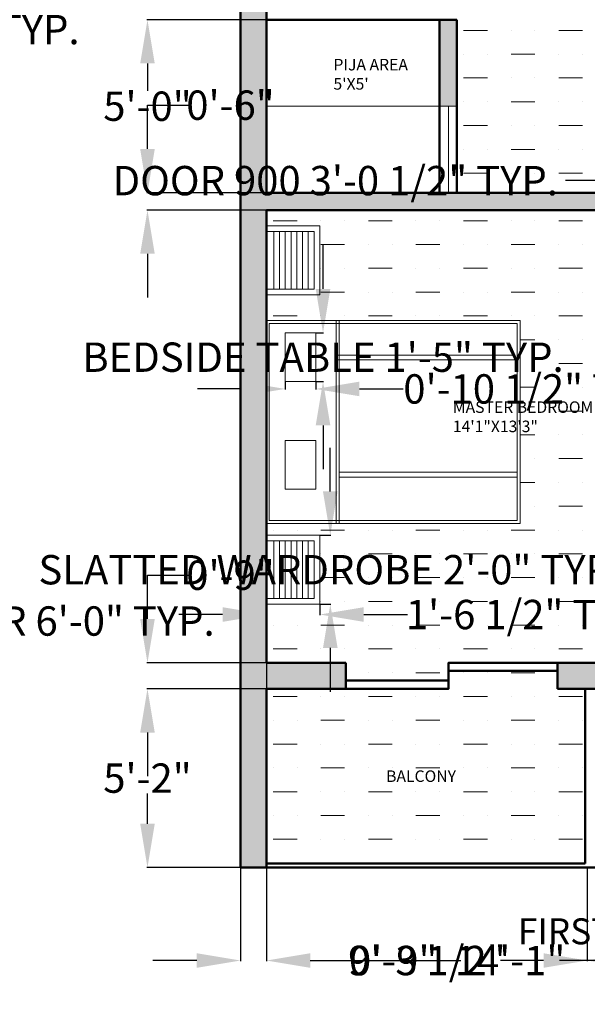
# Model space of a CAD drawing. Units: inches. Extents: x 26 to 14419, y 2 to 3479.
# Tile 6 of 9: x 14003 to 14200, y 2764 to 3106. Entities that reach past the tile are written whole.
import ezdxf

# ---------------------------------------------------------------- set-up
doc = ezdxf.new("R2010")
doc.units = ezdxf.units.IN
doc.header["$MEASUREMENT"] = 0
for name, color, linetype, lineweight in [('A-ANNO-DIMS', 2, 'Continuous', 18), ('A-ANNO-TEXT', 7, 'Continuous', 25), ('A-AREA-IDEN', 7, 'Continuous', 18), ('A-FLOR-PATT', 252, 'Continuous', 13), ('A-FURN', 8, 'Continuous', 18), ('A-WALL', 7, 'Continuous', 50)]:
    doc.layers.add(name, color=color, linetype=linetype, lineweight=lineweight)
doc.styles.get("Standard").update_dxf_attribs({"font": 'arial.ttf'})
doc.dimstyles.get("Standard").update_dxf_attribs({"dimtxt": 10.18, "dimasz": 15.18, "dimexe": 0.18, "dimexo": 0.0625, "dimgap": 0.09, "dimtad": 0, "dimtih": 1, "dimtoh": 1, "dimdec": 0, "dimzin": 0, "dimdsep": 46, "dimlunit": 3, "dimtxsty": 'Standard', "dimcen": 0.09, "dimadec": 0, "dimazin": 0, "dimtfac": 1, "dimtdec": 0, "dimtofl": 0, "dimtmove": 0, "dimatfit": 3, "dimfxl": 1, "dimtolj": 1, "dimtzin": 0, "dimarcsym": 0})

# ---------------------------------------------------------------- blocks, each defined once
blk = doc.blocks.new('WARDROBE-SLAT')
for p, q in [((2.53, 21.91), (2.53, 2)), ((4.53, 21.91), (4.53, 2)), ((6.53, 21.91), (6.53, 2)), ((8.53, 21.91), (8.53, 2)), ((10.53, 21.91), (10.53, 2)), ((12.53, 21.91), (12.53, 2)), ((14.53, 21.91), (14.53, 2))]:
    blk.add_line(p, q)
blk.add_lwpolyline([(0, 23.91), (18.56, 23.91), (18.56, 0), (0, 0)])
blk.add_lwpolyline([(0, 21.91), (16.56, 21.91), (16.56, 2), (0, 2)], close=True)
blk = doc.blocks.new('BEDSIDE-TABLE')
blk.add_lwpolyline([(0, 16.94), (10.58, 16.94), (10.58, 0), (0, 0)], close=True)
blk = doc.blocks.new('*D25')
at = {"layer": 'A-ANNO-DIMS', "color": 0, "lineweight": -2, "transparency": 16777216}
for p, q in [((14212.95, 3101.37), (14207.39, 3101.37)), ((14207.57, 3086.19), (14207.57, 3080.27)), ((14212.95, 3065.09), (14207.39, 3065.09)), ((14207.57, 3065.09), (14207.57, 3049.91)), ((14207.57, 3049.91), (14192.39, 3049.91))]:
    blk.add_line(p, q, dxfattribs=at)
at = {"layer": 'A-ANNO-DIMS', "color": 0, "transparency": 16777216}
for points in [[(14205.04, 3086.19), (14210.1, 3086.19), (14207.57, 3101.37)], [(14205.04, 3080.27), (14210.1, 3080.27), (14207.57, 3065.09)]]:
    blk.add_solid(points, dxfattribs=at)
at = {"layer": 'Defpoints', "color": 0, "transparency": 16777216}
for p in [(14213.01, 3101.37), (14207.57, 3065.09), (14213.01, 3065.09)]:
    blk.add_point(p, dxfattribs=at)
at = {"layer": 'A-ANNO-DIMS', "color": 0, "transparency": 16777216, "insert": (14112.52, 3049.91), "char_height": 10.18, "attachment_point": 5}
blk.add_mtext('\\A1;DOOR 900 3\'-0 1/2" TYP.', dxfattribs=at)
blk = doc.blocks.new('*D29')
at = {"layer": 'A-ANNO-DIMS', "color": 0, "lineweight": -2, "transparency": 16777216}
for p, q in [((13817.09, 2907.93), (13817.09, 2897.02)), ((13889.09, 2907.93), (13889.09, 2897.02)), ((13832.27, 2897.2), (13873.91, 2897.2)), ((13889.09, 2897.2), (13904.27, 2897.2))]:
    blk.add_line(p, q, dxfattribs=at)
at = {"layer": 'A-ANNO-DIMS', "color": 0, "transparency": 16777216}
for points in [[(13832.27, 2899.73), (13832.27, 2894.67), (13817.09, 2897.2)], [(13873.91, 2899.73), (13873.91, 2894.67), (13889.09, 2897.2)]]:
    blk.add_solid(points, dxfattribs=at)
at = {"layer": 'Defpoints', "color": 0, "transparency": 16777216}
for p in [(13817.09, 2908), (13889.09, 2908), (13889.09, 2897.2)]:
    blk.add_point(p, dxfattribs=at)
at = {"layer": 'A-ANNO-DIMS', "color": 0, "transparency": 16777216, "insert": (13989.66, 2897.2), "char_height": 10.18, "attachment_point": 5}
blk.add_mtext('\\A1;DOUBLE DOOR 6\'-0" TYP.', dxfattribs=at)
blk = doc.blocks.new('*D39')
at = {"layer": 'A-ANNO-DIMS', "color": 0, "lineweight": -2, "transparency": 16777216}
for p, q in [((14110.79, 2942.13), (14110.79, 2957.31)), ((14107.27, 2926.95), (14110.97, 2926.95)), ((14107.27, 2903.04), (14110.97, 2903.04)), ((14110.79, 2887.86), (14110.79, 2872.68))]:
    blk.add_line(p, q, dxfattribs=at)
at = {"layer": 'A-ANNO-DIMS', "color": 0, "transparency": 16777216}
for points in [[(14108.26, 2942.13), (14113.32, 2942.13), (14110.79, 2926.95)], [(14108.26, 2887.86), (14113.32, 2887.86), (14110.79, 2903.04)]]:
    blk.add_solid(points, dxfattribs=at)
at = {"layer": 'Defpoints', "color": 0, "transparency": 16777216}
for p in [(14107.2, 2926.95), (14110.79, 2926.95), (14107.2, 2903.04)]:
    blk.add_point(p, dxfattribs=at)
at = {"layer": 'A-ANNO-DIMS', "color": 0, "transparency": 16777216, "insert": (14110.79, 2914.99), "char_height": 10.18, "attachment_point": 5}
blk.add_mtext('\\A1;SLATTED WARDROBE 2\'-0" TYP.', dxfattribs=at)
blk = doc.blocks.new('*D40')
at = {"layer": 'A-ANNO-DIMS', "color": 0, "lineweight": -2, "transparency": 16777216}
for p, q in [((14088.64, 2902.97), (14088.64, 2899.27)), ((14107.2, 2902.97), (14107.2, 2899.27)), ((14073.46, 2899.45), (14058.28, 2899.45)), ((14122.38, 2899.45), (14137.56, 2899.45))]:
    blk.add_line(p, q, dxfattribs=at)
at = {"layer": 'A-ANNO-DIMS', "color": 0, "transparency": 16777216}
for points in [[(14073.46, 2901.98), (14073.46, 2896.92), (14088.64, 2899.45)], [(14122.38, 2901.98), (14122.38, 2896.92), (14107.2, 2899.45)]]:
    blk.add_solid(points, dxfattribs=at)
at = {"layer": 'Defpoints', "color": 0, "transparency": 16777216}
for p in [(14088.64, 2903.04), (14107.2, 2903.04), (14107.2, 2899.45)]:
    blk.add_point(p, dxfattribs=at)
at = {"layer": 'A-ANNO-DIMS', "color": 0, "transparency": 16777216, "insert": (14180.06, 2899.45), "char_height": 10.18, "attachment_point": 5}
blk.add_mtext('\\A1;1\'-6 1/2" TYP.', dxfattribs=at)
blk = doc.blocks.new('*D43')
at = {"layer": 'A-ANNO-DIMS', "color": 0, "lineweight": -2, "transparency": 16777216}
for p, q in [((14108.27, 3012.34), (14108.27, 3027.52)), ((14105.79, 2997.16), (14108.45, 2997.16)), ((14105.79, 2980.22), (14108.45, 2980.22)), ((14108.27, 2965.04), (14108.27, 2949.86))]:
    blk.add_line(p, q, dxfattribs=at)
at = {"layer": 'A-ANNO-DIMS', "color": 0, "transparency": 16777216}
for points in [[(14105.74, 3012.34), (14110.8, 3012.34), (14108.27, 2997.16)], [(14105.74, 2965.04), (14110.8, 2965.04), (14108.27, 2980.22)]]:
    blk.add_solid(points, dxfattribs=at)
at = {"layer": 'Defpoints', "color": 0, "transparency": 16777216}
for p in [(14105.73, 2997.16), (14108.27, 2997.16), (14105.73, 2980.22)]:
    blk.add_point(p, dxfattribs=at)
at = {"layer": 'A-ANNO-DIMS', "color": 0, "transparency": 16777216, "insert": (14108.27, 2988.69), "char_height": 10.18, "attachment_point": 5}
blk.add_mtext('\\A1;BEDSIDE TABLE 1\'-5" TYP.', dxfattribs=at)
blk = doc.blocks.new('*D44')
at = {"layer": 'A-ANNO-DIMS', "color": 0, "lineweight": -2, "transparency": 16777216}
for p, q in [((14079.96, 2977.68), (14064.78, 2977.68)), ((14095.14, 2980.15), (14095.14, 2977.5)), ((14105.73, 2980.15), (14105.73, 2977.5)), ((14120.91, 2977.68), (14136.09, 2977.68))]:
    blk.add_line(p, q, dxfattribs=at)
at = {"layer": 'A-ANNO-DIMS', "color": 0, "transparency": 16777216}
for points in [[(14079.96, 2980.21), (14079.96, 2975.15), (14095.14, 2977.68)], [(14120.91, 2980.21), (14120.91, 2975.15), (14105.73, 2977.68)]]:
    blk.add_solid(points, dxfattribs=at)
at = {"layer": 'Defpoints', "color": 0, "transparency": 16777216}
for p in [(14095.14, 2980.22), (14105.73, 2980.22), (14105.73, 2977.68)]:
    blk.add_point(p, dxfattribs=at)
at = {"layer": 'A-ANNO-DIMS', "color": 0, "transparency": 16777216, "insert": (14183.02, 2977.68), "char_height": 10.18, "attachment_point": 5}
blk.add_mtext('\\A1;0\'-10 1/2" TYP.', dxfattribs=at)
blk = doc.blocks.new('*D46')
at = {"layer": 'A-ANNO-DIMS', "color": 0, "lineweight": -2, "transparency": 16777216}
for p, q in [((13893.41, 3104.57), (13893.41, 3102.12)), ((13907.93, 3104.57), (13907.93, 3102.12)), ((13878.23, 3102.3), (13863.05, 3102.3)), ((13923.11, 3102.3), (13938.29, 3102.3))]:
    blk.add_line(p, q, dxfattribs=at)
at = {"layer": 'A-ANNO-DIMS', "color": 0, "transparency": 16777216}
for points in [[(13878.23, 3104.83), (13878.23, 3099.77), (13893.41, 3102.3)], [(13923.11, 3104.83), (13923.11, 3099.77), (13907.93, 3102.3)]]:
    blk.add_solid(points, dxfattribs=at)
at = {"layer": 'Defpoints', "color": 0, "transparency": 16777216}
for p in [(13893.41, 3104.63), (13907.93, 3104.63), (13907.93, 3102.3)]:
    blk.add_point(p, dxfattribs=at)
at = {"layer": 'A-ANNO-DIMS', "color": 0, "transparency": 16777216, "insert": (13980.79, 3102.3), "char_height": 10.18, "attachment_point": 5}
blk.add_mtext('\\A1;1\'-2 1/2" TYP.', dxfattribs=at)
blk = doc.blocks.new('*D84')
at = {"layer": 'A-ANNO-DIMS', "color": 0, "lineweight": -2, "transparency": 16777216}
for p, q in [((14079.64, 2811.66), (14079.64, 2779.29)), ((14088.64, 2811.66), (14088.64, 2779.29)), ((14064.46, 2779.47), (14049.28, 2779.47)), ((14103.82, 2779.47), (14119, 2779.47))]:
    blk.add_line(p, q, dxfattribs=at)
at = {"layer": 'A-ANNO-DIMS', "color": 0, "transparency": 16777216}
for points in [[(14064.46, 2782), (14064.46, 2776.94), (14079.64, 2779.47)], [(14103.82, 2782), (14103.82, 2776.94), (14088.64, 2779.47)]]:
    blk.add_solid(points, dxfattribs=at)
at = {"layer": 'Defpoints', "color": 0, "transparency": 16777216}
for p in [(14079.64, 2811.72), (14088.64, 2811.72), (14088.64, 2779.47)]:
    blk.add_point(p, dxfattribs=at)
at = {"layer": 'A-ANNO-DIMS', "color": 0, "transparency": 16777216, "insert": (14132.62, 2779.47), "char_height": 10.18, "attachment_point": 5}
blk.add_mtext('\\A1;0\'-9"', dxfattribs=at)
blk = doc.blocks.new('*D85')
at = {"layer": 'A-ANNO-DIMS', "color": 0, "lineweight": -2, "transparency": 16777216}
for p, q in [((14088.64, 2811.66), (14088.64, 2779.29)), ((14199.93, 2811.66), (14199.93, 2779.29)), ((14103.82, 2779.47), (14118.8, 2779.47)), ((14184.75, 2779.47), (14169.77, 2779.47))]:
    blk.add_line(p, q, dxfattribs=at)
at = {"layer": 'A-ANNO-DIMS', "color": 0, "transparency": 16777216}
for points in [[(14103.82, 2782), (14103.82, 2776.94), (14088.64, 2779.47)], [(14184.75, 2782), (14184.75, 2776.94), (14199.93, 2779.47)]]:
    blk.add_solid(points, dxfattribs=at)
at = {"layer": 'Defpoints', "color": 0, "transparency": 16777216}
for p in [(14088.64, 2811.72), (14199.93, 2811.72), (14199.93, 2779.47)]:
    blk.add_point(p, dxfattribs=at)
at = {"layer": 'A-ANNO-DIMS', "color": 0, "transparency": 16777216, "insert": (14144.28, 2779.47), "char_height": 10.18, "attachment_point": 5}
blk.add_mtext('\\A1;9\'-3 1/2"', dxfattribs=at)
blk = doc.blocks.new('*D86')
at = {"layer": 'A-ANNO-DIMS', "color": 0, "lineweight": -2, "transparency": 16777216}
for p, q in [((14199.93, 2811.66), (14199.93, 2779.29)), ((14333.64, 2811.66), (14333.64, 2779.29)), ((14215.11, 2779.47), (14237.83, 2779.47)), ((14318.46, 2779.47), (14295.74, 2779.47))]:
    blk.add_line(p, q, dxfattribs=at)
at = {"layer": 'A-ANNO-DIMS', "color": 0, "transparency": 16777216}
for points in [[(14215.11, 2782), (14215.11, 2776.94), (14199.93, 2779.47)], [(14318.46, 2782), (14318.46, 2776.94), (14333.64, 2779.47)]]:
    blk.add_solid(points, dxfattribs=at)
at = {"layer": 'Defpoints', "color": 0, "transparency": 16777216}
for p in [(14199.93, 2811.72), (14333.64, 2811.72), (14333.64, 2779.47)]:
    blk.add_point(p, dxfattribs=at)
at = {"layer": 'A-ANNO-DIMS', "color": 0, "transparency": 16777216, "insert": (14266.78, 2779.47), "char_height": 10.18, "attachment_point": 5}
blk.add_mtext('\\A1;11\'-1 1/2"', dxfattribs=at)
blk = doc.blocks.new('*D88')
at = {"layer": 'A-ANNO-DIMS', "color": 0, "lineweight": -2, "transparency": 16777216}
for p, q in [((14088.58, 2873.72), (14047.21, 2873.72)), ((14047.39, 2858.54), (14047.39, 2848.01)), ((14047.39, 2826.9), (14047.39, 2837.43)), ((14088.58, 2811.72), (14047.21, 2811.72))]:
    blk.add_line(p, q, dxfattribs=at)
at = {"layer": 'A-ANNO-DIMS', "color": 0, "transparency": 16777216}
for points in [[(14044.86, 2858.54), (14049.92, 2858.54), (14047.39, 2873.72)], [(14044.86, 2826.9), (14049.92, 2826.9), (14047.39, 2811.72)]]:
    blk.add_solid(points, dxfattribs=at)
at = {"layer": 'Defpoints', "color": 0, "transparency": 16777216}
for p in [(14047.39, 2873.72), (14088.64, 2873.72), (14088.64, 2811.72)]:
    blk.add_point(p, dxfattribs=at)
at = {"layer": 'A-ANNO-DIMS', "color": 0, "transparency": 16777216, "insert": (14047.39, 2842.72), "char_height": 10.18, "attachment_point": 5}
blk.add_mtext('\\A1;5\'-2"', dxfattribs=at)
blk = doc.blocks.new('*D89')
at = {"layer": 'A-ANNO-DIMS', "color": 0, "lineweight": -2, "transparency": 16777216}
for p, q in [((14047.39, 2897.9), (14047.39, 2913.08)), ((14047.39, 2913.08), (14062.57, 2913.08)), ((14088.58, 2882.72), (14047.21, 2882.72)), ((14088.58, 2873.72), (14047.21, 2873.72)), ((14047.39, 2858.54), (14047.39, 2843.36))]:
    blk.add_line(p, q, dxfattribs=at)
at = {"layer": 'A-ANNO-DIMS', "color": 0, "transparency": 16777216}
for points in [[(14044.86, 2897.9), (14049.92, 2897.9), (14047.39, 2882.72)], [(14044.86, 2858.54), (14049.92, 2858.54), (14047.39, 2873.72)]]:
    blk.add_solid(points, dxfattribs=at)
at = {"layer": 'Defpoints', "color": 0, "transparency": 16777216}
for p in [(14047.39, 2882.72), (14088.64, 2882.72), (14088.64, 2873.72)]:
    blk.add_point(p, dxfattribs=at)
at = {"layer": 'A-ANNO-DIMS', "color": 0, "transparency": 16777216, "insert": (14076.19, 2913.08), "char_height": 10.18, "attachment_point": 5}
blk.add_mtext('\\A1;0\'-9"', dxfattribs=at)
blk = doc.blocks.new('*D91')
at = {"layer": 'A-ANNO-DIMS', "color": 0, "lineweight": -2, "transparency": 16777216}
for p, q in [((14047.39, 3060.9), (14047.39, 3076.08)), ((14047.39, 3076.08), (14062.57, 3076.08)), ((14088.58, 3045.72), (14047.21, 3045.72)), ((14088.58, 3039.72), (14047.21, 3039.72)), ((14047.39, 3024.54), (14047.39, 3009.36))]:
    blk.add_line(p, q, dxfattribs=at)
at = {"layer": 'A-ANNO-DIMS', "color": 0, "transparency": 16777216}
for points in [[(14044.86, 3060.9), (14049.92, 3060.9), (14047.39, 3045.72)], [(14044.86, 3024.54), (14049.92, 3024.54), (14047.39, 3039.72)]]:
    blk.add_solid(points, dxfattribs=at)
at = {"layer": 'Defpoints', "color": 0, "transparency": 16777216}
for p in [(14047.39, 3045.72), (14088.64, 3045.72), (14088.64, 3039.72)]:
    blk.add_point(p, dxfattribs=at)
at = {"layer": 'A-ANNO-DIMS', "color": 0, "transparency": 16777216, "insert": (14076.19, 3076.08), "char_height": 10.18, "attachment_point": 5}
blk.add_mtext('\\A1;0\'-6"', dxfattribs=at)
blk = doc.blocks.new('*D92')
at = {"layer": 'A-ANNO-DIMS', "color": 0, "lineweight": -2, "transparency": 16777216}
for p, q in [((14088.58, 3105.72), (14047.21, 3105.72)), ((14047.39, 3090.54), (14047.39, 3081.01)), ((14047.39, 3060.9), (14047.39, 3070.43)), ((14088.58, 3045.72), (14047.21, 3045.72))]:
    blk.add_line(p, q, dxfattribs=at)
at = {"layer": 'A-ANNO-DIMS', "color": 0, "transparency": 16777216}
for points in [[(14044.86, 3090.54), (14049.92, 3090.54), (14047.39, 3105.72)], [(14044.86, 3060.9), (14049.92, 3060.9), (14047.39, 3045.72)]]:
    blk.add_solid(points, dxfattribs=at)
at = {"layer": 'Defpoints', "color": 0, "transparency": 16777216}
for p in [(14047.39, 3105.72), (14088.64, 3105.72), (14088.64, 3045.72)]:
    blk.add_point(p, dxfattribs=at)
at = {"layer": 'A-ANNO-DIMS', "color": 0, "transparency": 16777216, "insert": (14047.39, 3075.72), "char_height": 10.18, "attachment_point": 5}
blk.add_mtext('\\A1;5\'-0"', dxfattribs=at)
blk = doc.blocks.new('*D110')
at = {"layer": 'A-ANNO-DIMS', "color": 0, "lineweight": -2, "transparency": 16777216}
for p, q in [((14088.64, 2882.66), (14088.64, 2779.29)), ((14257.64, 2882.66), (14257.64, 2779.29)), ((14103.82, 2779.47), (14156.05, 2779.47)), ((14242.46, 2779.47), (14190.24, 2779.47))]:
    blk.add_line(p, q, dxfattribs=at)
at = {"layer": 'A-ANNO-DIMS', "color": 0, "transparency": 16777216}
for points in [[(14103.82, 2782), (14103.82, 2776.94), (14088.64, 2779.47)], [(14242.46, 2782), (14242.46, 2776.94), (14257.64, 2779.47)]]:
    blk.add_solid(points, dxfattribs=at)
at = {"layer": 'Defpoints', "color": 0, "transparency": 16777216}
for p in [(14088.64, 2882.72), (14257.64, 2882.72), (14257.64, 2779.47)]:
    blk.add_point(p, dxfattribs=at)
at = {"layer": 'A-ANNO-DIMS', "color": 0, "transparency": 16777216, "insert": (14173.14, 2779.47), "char_height": 10.18, "attachment_point": 5}
blk.add_mtext('\\A1;14\'-1"', dxfattribs=at)

msp = doc.modelspace()

# ---------------------------------------------------------------- hatches: boundary and pattern name
at = {"layer": 'A-FLOR-PATT'}
h = msp.add_hatch(color=256, dxfattribs=at)
h.dxf.hatch_style = 1
h.paths.add_polyline_path([(13922.09, 3432), (13659.09, 3432), (13659.09, 2842), (13668.09, 2842), (13668.09, 2851), (13668.09, 2899), (13668.09, 2908), (13668.09, 3076), (13706.09, 3076), (13706.09, 3085), (13668.09, 3085), (13668.09, 3249), (13712.76, 3249), (13712.76, 3255), (13668.09, 3255), (13668.09, 3375), (13720.94, 3375), (13720.94, 3378, -0.017236), (13720.94, 3380), (13720.94, 3381), (13668.09, 3381), (13668.09, 3423), (13784.09, 3423), (13784.09, 3381), (13753.94, 3381), (13753.94, 3375), (13784.09, 3375), (13784.09, 3255), (13758.77, 3255), (13758.77, 3249), (13784.09, 3249), (13793.09, 3249), (13793.09, 3255), (13793.09, 3423), (13913.09, 3423), (13913.09, 3255), (13832.09, 3255), (13832.09, 3254, -0.014283), (13832.09, 3252), (13832.09, 3249), (13836.57, 3249), (13836.57, 3234), (13839.57, 3234, -0.017236), (13841.57, 3234), (13842.57, 3234), (13842.57, 3249), (13913.09, 3249), (13913.09, 3201), (13892.46, 3201), (13793.09, 3201), (13784.09, 3201), (13784.09, 3195), (13793.09, 3195), (13913.09, 3195), (13913.09, 3127), (13922.09, 3127)])
h.paths.add_polyline_path([(13922.09, 3013.5), (13913.09, 3013.5), (13913.09, 2908), (13892.09, 2908), (13892.09, 2899), (13913.09, 2899), (13913.09, 2851), (13793.09, 2851), (13784.09, 2851), (13784.09, 2842), (13922.09, 2842)], flags=17)
h.paths.add_polyline_path([(13793.09, 3085), (13784.09, 3085), (13784.09, 3076), (13784.09, 3071.08), (13784.09, 3066.17), (13784.09, 2908), (13784.09, 2899.07), (13793.09, 2899), (13802.09, 2899), (13814.09, 2899), (13814.09, 2908), (13793.09, 2908)], flags=17)
h.paths.add_polyline_path([(14342.64, 3401.72), (14242.78, 3401.72), (14242.78, 3392.72), (14257.64, 3392.72), (14257.64, 3351.75), (14257.64, 3345.75), (14257.64, 3330.73), (14263.64, 3330.73), (14263.64, 3392.72), (14333.64, 3392.72), (14333.64, 3284.72), (14302.92, 3284.72), (14302.92, 3281.72, -0.022645), (14302.92, 3279.12), (14302.92, 3278.72), (14333.64, 3278.72), (14333.64, 3170.72), (14316.1, 3170.72), (14263.64, 3170.72), (14263.64, 3278.72), (14269.92, 3278.72), (14269.92, 3284.72), (14263.64, 3284.72), (14257.64, 3284.72), (14257.64, 3225.75), (14257.64, 3219.75), (14257.64, 3164.72), (14333.64, 3164.72), (14333.64, 3110.37), (14210.01, 3110.37), (14210.01, 3104.37), (14257.64, 3104.37), (14257.64, 3024), (14263.64, 3024), (14263.64, 3039.72), (14263.64, 3104.37), (14333.64, 3104.37), (14333.64, 3045.72), (14333.64, 3039.72), (14333.64, 2967.72), (14296.64, 2967.72), (14296.64, 2964.72, -0.017236), (14296.64, 2962.72), (14296.64, 2961.72), (14333.64, 2961.72), (14333.64, 2882.72), (14312.64, 2882.72), (14312.64, 2873.72), (14333.64, 2873.72), (14333.64, 2820.72), (14333.64, 2811.72), (14342.64, 2811.72)])
h.paths.add_polyline_path([(14088.64, 3219.75), (14218.64, 3219.75), (14218.64, 3222.75, -0.014283), (14218.64, 3224.75), (14218.64, 3225.75), (14088.64, 3225.75), (14088.64, 3345.75), (14088.64, 3351.75), (14088.64, 3392.72), (14193.93, 3392.72), (14193.93, 3351.75), (14140.64, 3351.75), (14140.64, 3345.75), (14170.7, 3345.75), (14218.64, 3345.75), (14218.64, 3348.75, -0.014283), (14218.64, 3350.75), (14218.64, 3351.75), (14199.93, 3351.75), (14199.93, 3392.72), (14214.78, 3392.72), (14214.78, 3401.72), (14079.64, 3401.72), (14079.64, 2811.72), (14088.64, 2811.72), (14088.64, 2820.72), (14088.64, 2873.72), (14116.21, 2873.72), (14116.21, 2876.57), (14116.21, 2882.72), (14088.64, 2882.72), (14088.64, 3039.72), (14216.01, 3039.72), (14216.01, 3065.37), (14215.01, 3065.37, -0.014283), (14213.01, 3065.37), (14210.01, 3065.37), (14210.01, 3045.72), (14154.64, 3045.72), (14148.64, 3045.72), (14088.64, 3045.72)])
h.paths.add_polyline_path([(14284.64, 2882.72), (14263.64, 2882.72), (14263.64, 2961.72), (14263.64, 2967.72), (14257.64, 2967.72), (14257.64, 2956.69), (14257.64, 2916.18), (14257.64, 2882.72), (14249.61, 2882.72), (14249.61, 2873.72), (14284.64, 2873.72)], flags=17)
h.paths.add_polyline_path([(14202.78, 2882.72), (14189.55, 2882.72), (14189.55, 2879.95), (14189.55, 2873.72), (14202.78, 2873.72)], flags=17)
h = msp.add_hatch(dxfattribs=at)
h.set_pattern_fill('MUDST', color=256, scale=33)
h.paths.add_polyline_path([(14304.4, 3368.55), (14263.64, 3368.55), (14263.64, 3330.73), (14257.64, 3330.73), (14257.64, 3345.75), (14254.64, 3345.75), (14254.64, 3348.75), (14252.64, 3348.75), (14252.64, 3384.75, 0.397579), (14218.64, 3350.75), (14218.64, 3345.75), (14170.7, 3345.75), (14170.7, 3274.26), (14114.64, 3274.26), (14114.64, 3345.75), (14088.64, 3345.75), (14088.64, 3225.75), (14114.67, 3225.75), (14114.67, 3239.54), (14174.56, 3239.54), (14174.56, 3225.75), (14218.69, 3225.75, -0.405865), (14254.64, 3258.75), (14254.64, 3225.75), (14257.64, 3225.75), (14257.64, 3284.72), (14263.64, 3284.72), (14272.92, 3284.72), (14272.92, 3281.72), (14274.92, 3281.72), (14274.92, 3251.72, 0.394163), (14302.92, 3279.12), (14302.92, 3284.72), (14304.4, 3284.72)])
h.paths.add_polyline_path([(14189.03, 3330.51), (14176.21, 3330.51), (14176.21, 3342.77), (14189.03, 3342.77)], flags=16)
h.paths.add_polyline_path([(14188.03, 3331.51), (14177.21, 3331.51), (14177.21, 3341.77), (14188.03, 3341.77)], flags=0)
h.paths.add_polyline_path([(14185.02, 3336.64, -1), (14180.21, 3336.64, -1)], flags=0)
h.paths.add_polyline_path([(14109.33, 3330.51), (14096.5, 3330.51), (14096.5, 3342.77), (14109.33, 3342.77)], flags=16)
h.paths.add_polyline_path([(14108.33, 3331.51), (14097.5, 3331.51), (14097.5, 3341.77), (14108.33, 3341.77)], flags=0)
h.paths.add_polyline_path([(14105.32, 3336.64, -1), (14100.51, 3336.64, -1)], flags=0)
h.paths.add_polyline_path([(14257.64, 3219.75), (14254.64, 3219.75), (14254.64, 3222.75), (14252.64, 3222.75), (14252.64, 3258.75, 0.397579), (14218.64, 3224.75), (14218.64, 3219.75), (14088.64, 3219.75), (14088.64, 3105.72), (14154.64, 3105.72), (14154.64, 3045.72), (14210.01, 3045.72), (14210.01, 3065.37), (14215.01, 3065.37, 0.397579), (14249.01, 3099.37), (14213.01, 3099.37), (14213.01, 3101.37), (14210.01, 3101.37), (14210.01, 3110.37), (14217.64, 3110.37), (14217.64, 3164.72), (14215.11, 3164.72), (14215.11, 3170.72), (14257.64, 3170.72)])
h.paths.add_polyline_path([(14174.2, 3192.28), (14172.21, 3192.28), (14172.21, 3190.47), (14113.94, 3190.47), (14113.94, 3192.28), (14112.02, 3192.28), (14112.02, 3207.65), (14113.94, 3207.65), (14174.2, 3207.65)], flags=16)
h.paths.add_polyline_path([(14132.26, 3203.31), (14132.26, 3205.54), (14153.01, 3205.54), (14153.01, 3203.31)], flags=0)
h.paths.add_polyline_path([(14139.45, 3178.77), (14139.45, 3144.03), (14124.04, 3144.03), (14124.04, 3178.77)], flags=16)
h.paths.add_polyline_path([(14138.45, 3177.77), (14138.45, 3145.03), (14125.04, 3145.03), (14125.04, 3177.77)], flags=0)
h.paths.add_polyline_path([(14127.62, 3154.26), (14127.69, 3154.32), (14127.65, 3154.8), (14127.17, 3154.71)], flags=0)
h.paths.add_polyline_path([(14137.62, 3155.43), (14138.07, 3155.38), (14137.86, 3155.74)], flags=0)
h.paths.add_polyline_path([(14134.11, 3152.76), (14134.62, 3152.52), (14134.75, 3152.98)], flags=0)
h.paths.add_polyline_path([(14134.97, 3149.61), (14135.06, 3149.3), (14135.3, 3149.21), (14134.97, 3149.61)], flags=0)
h.paths.add_polyline_path([(14129.06, 3148.22), (14128.85, 3148.19), (14128.88, 3147.91)], flags=0)
h.paths.add_polyline_path([(14129.76, 3149.73), (14129.77, 3149.7), (14129.81, 3149.73)], flags=0)
h.paths.add_polyline_path([(14129.81, 3152.94), (14129.51, 3152.8), (14129.91, 3152.74)], flags=0)
h.paths.add_polyline_path([(14129.97, 3154.13), (14131.4, 3152.09), (14132.47, 3152.75), (14132.58, 3152.96)], flags=0)
h.paths.add_polyline_path([(14131.76, 3158.63), (14131.62, 3158.74), (14131.67, 3158.49)], flags=0)
h.paths.add_polyline_path([(14133.11, 3151.99), (14133.11, 3152.01), (14133.11, 3151.99)], flags=0)
h.paths.add_polyline_path([(14135.18, 3148.48), (14135.04, 3148), (14135.53, 3147.73), (14135.69, 3148.25)], flags=0)
h.paths.add_polyline_path([(14111.74, 3127.44), (14109.92, 3127.44), (14109.92, 3125.52), (14094.56, 3125.52), (14094.56, 3127.44), (14094.56, 3187.7), (14109.92, 3187.7), (14109.92, 3185.71), (14111.74, 3185.71)], flags=16)
h.paths.add_polyline_path([(14098.89, 3166.51), (14098.89, 3145.76), (14096.67, 3145.76), (14096.67, 3166.51)], flags=0)
h.paths.add_polyline_path([(14107.98, 3191.64), (14092.66, 3191.64), (14092.66, 3205.45), (14107.98, 3205.45)], flags=16)
h.paths.add_polyline_path([(14102.61, 3192.64), (14102.72, 3192.57), (14102.74, 3192.64)], flags=0)
h.paths.add_polyline_path([(14101.15, 3198.79), (14101.66, 3198.55), (14101.79, 3199)], flags=0)
h.paths.add_polyline_path([(14105.37, 3201.99), (14105.29, 3202.26), (14105.04, 3201.95)], flags=0)
h.paths.add_polyline_path([(14102.01, 3195.63), (14102.11, 3195.33), (14102.34, 3195.23), (14102.02, 3195.64)], flags=0)
h.paths.add_polyline_path([(14102.22, 3194.5), (14102.08, 3194.03), (14102.57, 3193.75), (14102.73, 3194.27)], flags=0)
h.paths.add_polyline_path([(14096.1, 3194.24), (14095.89, 3194.22), (14095.92, 3193.93)], flags=0)
h.paths.add_polyline_path([(14096.81, 3195.75), (14096.81, 3195.72), (14096.85, 3195.75)], flags=0)
h.paths.add_polyline_path([(14094.74, 3200.21), (14094.69, 3200.82), (14094.21, 3200.74)], flags=0)
h.paths.add_polyline_path([(14096.86, 3198.97), (14096.55, 3198.82), (14096.95, 3198.77)], flags=0)
h.paths.add_polyline_path([(14097.01, 3200.16), (14098.44, 3198.11), (14099.51, 3198.78), (14099.62, 3198.98)], flags=0)
h.paths.add_polyline_path([(14098.8, 3204.66), (14098.66, 3204.77), (14098.71, 3204.51)], flags=0)
h.paths.add_polyline_path([(14100.15, 3198.02), (14100.15, 3198.03), (14100.15, 3198.02)], flags=0)
h.paths.add_polyline_path([(14257.64, 2967.72), (14263.64, 2967.72), (14266.64, 2967.72), (14296.64, 2967.72), (14304.52, 2967.72), (14304.52, 3072.04), (14263.64, 3072.04), (14263.64, 3039.72), (14263.64, 3024), (14257.64, 3024), (14257.64, 3104.37), (14216.01, 3104.37), (14216.01, 3101.37), (14249.01, 3101.37, -0.405865), (14216.01, 3065.41), (14216.01, 3039.72), (14088.64, 3039.72), (14088.64, 3034.24), (14107.2, 3034.24), (14107.2, 3010.33), (14088.64, 3010.33), (14088.64, 3001.38), (14176.64, 3001.38), (14176.64, 2931.05), (14088.64, 2931.05), (14088.64, 2926.95), (14107.2, 2926.95), (14107.2, 2903.04), (14088.64, 2903.04), (14088.64, 2882.72), (14116.21, 2882.72), (14116.21, 2876.57), (14151.84, 2876.57), (14151.84, 2882.72), (14189.55, 2882.72), (14257.64, 2882.72), (14257.64, 2916.18), (14244.9, 2916.18), (14244.9, 2956.69), (14257.64, 2956.69)])
h.paths.add_polyline_path([(14199.2, 2873.72), (14189.55, 2873.72), (14189.55, 2879.95), (14151.84, 2879.95), (14151.84, 2873.72), (14116.21, 2873.72), (14088.64, 2873.72), (14088.64, 2820.72), (14088.64, 2813.09), (14199.2, 2813.09)])
h.paths.add_polyline_path([(14272.13, 3336.81), (14293.39, 3336.81), (14293.39, 3351.73), (14272.13, 3351.73)], flags=24)
h.paths.add_polyline_path([(14208.53, 3375.98), (14237.24, 3375.98), (14237.24, 3384.22), (14208.53, 3384.22)], flags=25)
h.paths.add_polyline_path([(14136.68, 3250.57), (14220.54, 3250.57), (14220.54, 3272.96), (14136.68, 3272.96)], flags=24)
h.paths.add_polyline_path([(14121.4, 3116.81), (14182.4, 3116.81), (14182.4, 3131.73), (14121.4, 3131.73)], flags=24)
h.paths.add_polyline_path([(14268.29, 3033.43), (14289.54, 3033.43), (14289.54, 3048.36), (14268.29, 3048.36)], flags=24)
h.paths.add_polyline_path([(14151.68, 2960.42), (14207.58, 2960.42), (14207.58, 2975.35), (14151.68, 2975.35)], flags=25)
h.paths.add_polyline_path([(14128.74, 2839.15), (14157.44, 2839.15), (14157.44, 2847.39), (14128.74, 2847.39)], flags=24)
h = msp.add_hatch(color=256, dxfattribs=at)
h.dxf.hatch_style = 1
h.paths.add_polyline_path([(14154.64, 3105.72), (14148.64, 3105.72), (14148.64, 3075.72), (14154.64, 3075.72)])

# ---------------------------------------------------------------- linework, layer by layer
at = {"layer": 'A-FURN'}
for p, q in [((14154.64, 3075.72), (14088.64, 3075.72)), ((14151.83, 3075.72), (14151.83, 3045.72)), ((14112.86, 3001.38), (14112.86, 2931.05)), ((14113.86, 3001.38), (14113.86, 2931.05)), ((14112.86, 2989.42), (14174.64, 2989.42)), ((14112.86, 2987.76), (14174.64, 2987.76)), ((14113.86, 2948.77), (14175.64, 2948.77)), ((14113.86, 2947.12), (14175.64, 2947.12))]:
    msp.add_line(p, q, dxfattribs=at)
for points in [[(14088.64, 3001.38), (14176.64, 3001.38), (14176.64, 2931.05), (14088.64, 2931.05)], [(14089.64, 3000.38), (14175.64, 3000.38), (14175.64, 2932.05), (14089.64, 2932.05)]]:
    msp.add_lwpolyline(points, close=True, dxfattribs=at)
at = {"layer": 'A-WALL'}
for p, q in [((14079.64, 2811.72), (14079.64, 3401.72)), ((14088.64, 3045.72), (14088.64, 3219.75)), ((14154.64, 3105.72), (14088.64, 3105.72)), ((14148.64, 3045.72), (14148.64, 3105.72)), ((14154.64, 3045.72), (14154.64, 3105.72)), ((14148.64, 3045.72), (14088.64, 3045.72)), ((14154.64, 3045.72), (14148.64, 3045.72)), ((14210.01, 3045.72), (14154.64, 3045.72)), ((14088.64, 2882.72), (14088.64, 3039.72)), ((14216.01, 3039.72), (14088.64, 3039.72)), ((14116.21, 2882.72), (14088.64, 2882.72)), ((14116.21, 2882.72), (14116.21, 2873.72)), ((14257.64, 2882.72), (14151.84, 2882.72)), ((14189.55, 2882.72), (14189.55, 2873.72)), ((14088.64, 2820.72), (14088.64, 2873.72)), ((14151.84, 2873.72), (14088.64, 2873.72)), ((14333.64, 2873.72), (14189.55, 2873.72)), ((14199.2, 2813.09), (14199.2, 2873.72)), ((14088.64, 2820.72), (14088.64, 2811.72)), ((14342.64, 2811.72), (14079.64, 2811.72)), ((14199.2, 2813.09), (14088.64, 2813.09))]:
    msp.add_line(p, q, dxfattribs=at)
msp.add_lwpolyline([(14151.84, 2873.72), (14151.84, 2882.72)], dxfattribs=at)
for points in [[(14189.55, 2882.72), (14151.84, 2882.72), (14151.84, 2879.95), (14189.55, 2879.95)], [(14116.21, 2873.72), (14151.84, 2873.72), (14151.84, 2876.57), (14116.21, 2876.57)]]:
    msp.add_lwpolyline(points, close=True, dxfattribs=at)

# ---------------------------------------------------------------- block references
at = {"layer": 'A-FURN'}
for name, p in [('WARDROBE-SLAT', (14088.64, 3010.33)), ('BEDSIDE-TABLE', (14095.15, 2980.22)), ('BEDSIDE-TABLE', (14095.15, 2942.88)), ('WARDROBE-SLAT', (14088.64, 2903.04))]:
    msp.add_blockref(name, p, dxfattribs=at)

# ---------------------------------------------------------------- texts
at = {"layer": 'A-ANNO-TEXT', "insert": (14175.82, 2794.09), "char_height": 9, "attachment_point": 1}
msp.add_mtext_dynamic_manual_height_columns('FIRST  FLOOR', width=157.7562, gutter_width=1, heights=[0], dxfattribs=at)
at = {"layer": 'A-AREA-IDEN', "char_height": 4, "attachment_point": 1}
for s, width, insert in [("PIJA AREA\\P5'X5'", 32.6659, (14111.89, 3092.13)), ('MASTER BEDROOM\\P14\'1"X13\'3"', 58.5539, (14153.29, 2973.36)), ('BALCONY', 7.6086, (14130.15, 2845.4))]:
    msp.add_mtext_dynamic_manual_height_columns(s, width=width, gutter_width=1, heights=[0], dxfattribs=dict(at, insert=insert))

# ---------------------------------------------------------------- dimensions: what is measured, and where the dimension line sits
at = {"layer": 'A-ANNO-DIMS'}
for base, p1, p2, text, picture, middle in [((13907.93, 3102.3), (13893.41, 3104.63), (13907.93, 3104.63), '<> TYP.', '*D46', (13980.79, 3102.3)), ((14105.73, 2977.68), (14095.14, 2980.22), (14105.73, 2980.22), '<> TYP.', '*D44', (14183.02, 2977.68)), ((13889.09, 2897.2), (13817.09, 2908), (13889.09, 2908), 'DOUBLE DOOR <> TYP.', '*D29', (13989.66, 2897.2)), ((14107.2, 2899.45), (14088.64, 2903.04), (14107.2, 2903.04), '<> TYP.', '*D40', (14180.06, 2899.45))]:
    dim = msp.add_linear_dim(base=base, p1=p1, p2=p2, text=text, dimstyle='Standard', override={"dimdec": 1, "dimrnd": 0, "dimzin": 1, "dimlunit": 4, "dimfrac": 2}, dxfattribs=at)
    dim.commit()
    dim.dimension.update_dxf_attribs({"geometry": picture, "text_midpoint": middle})
for base, p1, p2, picture, middle in [((14047.39, 3105.72), (14088.64, 3045.72), (14088.64, 3105.72), '*D92', (14047.39, 3075.72)), ((14047.39, 3045.72), (14088.64, 3039.72), (14088.64, 3045.72), '*D91', (14076.19, 3076.08)), ((14047.39, 2882.72), (14088.64, 2873.72), (14088.64, 2882.72), '*D89', (14076.19, 2913.08)), ((14047.39, 2873.72), (14088.64, 2811.72), (14088.64, 2873.72), '*D88', (14047.39, 2842.72))]:
    dim = msp.add_linear_dim(base=base, p1=p1, p2=p2, angle=90, dimstyle='Standard', override={"dimdec": 1, "dimlfac": 1, "dimrnd": 0, "dimzin": 1, "dimdsep": 46, "dimlunit": 4, "dimfrac": 2}, dxfattribs=at)
    dim.commit()
    dim.dimension.update_dxf_attribs({"geometry": picture, "text_midpoint": middle})
for base, p1, p2, angle, text, picture, middle in [((14207.57, 3065.09), (14213.01, 3101.37), (14213.01, 3065.09), 270, 'DOOR 900 <> TYP.', '*D25', (14112.52, 3049.91)), ((14108.27, 2997.16), (14105.73, 2980.22), (14105.73, 2997.16), 90, 'BEDSIDE TABLE <> TYP.', '*D43', (14108.27, 2988.69)), ((14110.79, 2926.95), (14107.2, 2903.04), (14107.2, 2926.95), 90, 'SLATTED WARDROBE <> TYP.', '*D39', (14110.79, 2914.99))]:
    dim = msp.add_linear_dim(base=base, p1=p1, p2=p2, angle=angle, text=text, dimstyle='Standard', override={"dimdec": 1, "dimrnd": 0, "dimzin": 1, "dimlunit": 4, "dimfrac": 2}, dxfattribs=at)
    dim.commit()
    dim.dimension.update_dxf_attribs({"geometry": picture, "text_midpoint": middle})
for base, p1, p2, picture, middle in [((14257.64, 2779.47), (14088.64, 2882.72), (14257.64, 2882.72), '*D110', (14173.14, 2779.47)), ((14088.64, 2779.47), (14079.64, 2811.72), (14088.64, 2811.72), '*D84', (14132.62, 2779.47)), ((14199.93, 2779.47), (14088.64, 2811.72), (14199.93, 2811.72), '*D85', (14144.28, 2779.47)), ((14333.64, 2779.47), (14199.93, 2811.72), (14333.64, 2811.72), '*D86', (14266.78, 2779.47))]:
    dim = msp.add_linear_dim(base=base, p1=p1, p2=p2, dimstyle='Standard', override={"dimdec": 1, "dimlfac": 1, "dimrnd": 0, "dimzin": 1, "dimdsep": 46, "dimlunit": 4, "dimfrac": 2}, dxfattribs=at)
    dim.commit()
    dim.dimension.update_dxf_attribs({"geometry": picture, "text_midpoint": middle})

doc.saveas('drawing.dxf')
